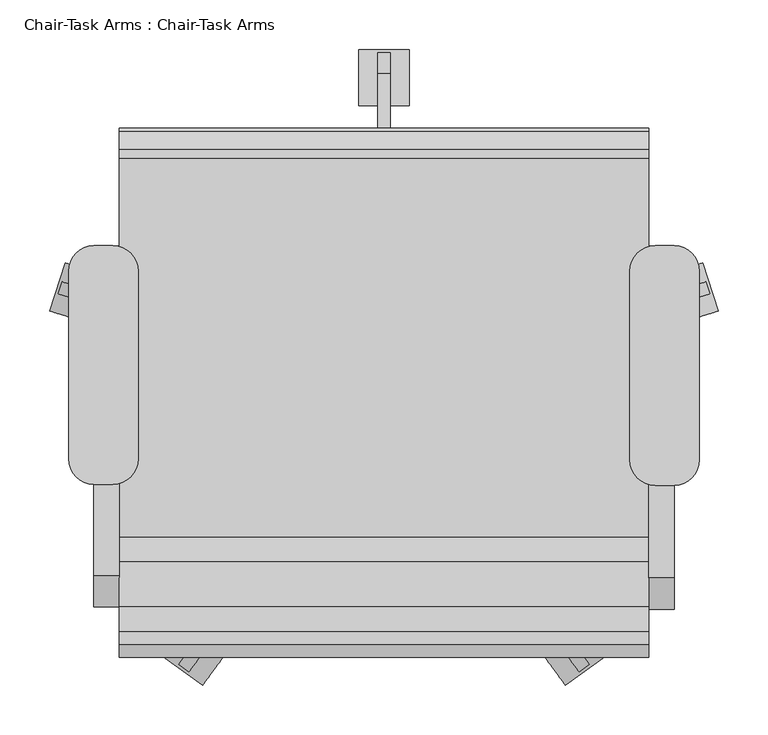
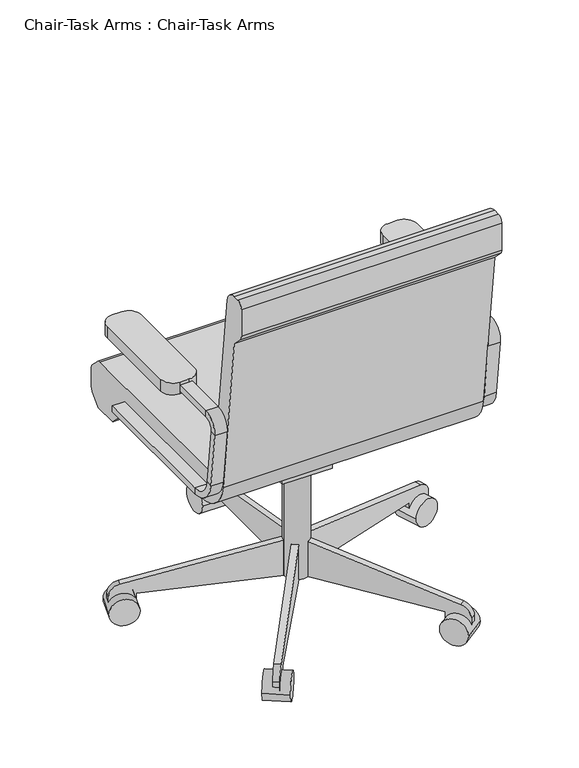
"""IFC4 building model written with IfcOpenShell, lengths in millimetres: furniture geometry, Chair-Task Arms : Chair-Task Arms."""

from ifc_helpers import new_model, si_unit, point, frame, frame_2d, origin, place, context, project, spatial, polyline, circle_curve, trimmed, segment, composite_curve, outline, extrude, source, transform, mapped, element, save
from ifc_brep_helpers import plane_surface, cylinder_surface, revolved_surface, advanced_brep


def chair_task_arms_chair_task_arms_fa5a08ef(model_context):
    return source(origin(), model_context, "Body", "SolidModel", [
        extrude(outline(composite_curve([segment(polyline([(433.0908197, -74.2028048), (414.0408197, -74.2028048)]), True, "CONTINUOUS"), segment(trimmed(circle_curve(frame_2d((414.0408197, -48.8028048)), 25.4), [point((414.0408197, -74.2028048))], [point((388.6408197, -48.8028048))], False, "CARTESIAN"), True, "CONTINUOUS"), segment(polyline([(388.6408197, -48.8028048), (388.6408197, 141.6319091)]), True, "CONTINUOUS"), segment(trimmed(circle_curve(frame_2d((414.0408197, 141.6319091)), 25.4), [point((388.6408197, 141.6319091))], [point((414.0408197, 167.0319091))], False, "CARTESIAN"), True, "CONTINUOUS"), segment(polyline([(414.0408197, 167.0319091), (433.0908197, 167.0319091)]), True, "CONTINUOUS"), segment(trimmed(circle_curve(frame_2d((433.0908197, 141.6319091)), 25.4), [point((433.0908197, 167.0319091))], [point((458.4908197, 141.6319091))], False, "CARTESIAN"), True, "CONTINUOUS"), segment(polyline([(458.4908197, 141.6319091), (458.4908197, -48.8028048)]), True, "CONTINUOUS"), segment(trimmed(circle_curve(frame_2d((433.0908197, -48.8028048)), 25.4), [point((458.4908197, -48.8028048))], [point((433.0908197, -74.2028048))], False, "CARTESIAN"), True, "CONTINUOUS")], self_intersect=False)), frame((0.0, 0.0, 596.9), z_axis=(0.0, 0.0, 1.0), x_axis=(1.0, 0.0, 0.0)), (0.0, 0.0, 1.0), 25.4),
        extrude(outline(composite_curve([segment(polyline([(-132.0591803, -73.1575984), (-151.1091803, -73.1575984)]), True, "CONTINUOUS"), segment(trimmed(circle_curve(frame_2d((-151.1091803, -47.7575984)), 25.4), [point((-151.1091803, -73.1575984))], [point((-176.5091803, -47.7575984))], False, "CARTESIAN"), True, "CONTINUOUS"), segment(polyline([(-176.5091803, -47.7575984), (-176.5091803, 141.6319091)]), True, "CONTINUOUS"), segment(trimmed(circle_curve(frame_2d((-151.1091803, 141.6319091)), 25.4), [point((-176.5091803, 141.6319091))], [point((-151.1091803, 167.0319091))], False, "CARTESIAN"), True, "CONTINUOUS"), segment(polyline([(-151.1091803, 167.0319091), (-132.0591803, 167.0319091)]), True, "CONTINUOUS"), segment(trimmed(circle_curve(frame_2d((-132.0591803, 141.6319091)), 25.4), [point((-132.0591803, 167.0319091))], [point((-106.6591803, 141.6319091))], False, "CARTESIAN"), True, "CONTINUOUS"), segment(polyline([(-106.6591803, 141.6319091), (-106.6591803, -47.7575984)]), True, "CONTINUOUS"), segment(trimmed(circle_curve(frame_2d((-132.0591803, -47.7575984)), 25.4), [point((-106.6591803, -47.7575984))], [point((-132.0591803, -73.1575984))], False, "CARTESIAN"), True, "CONTINUOUS")], self_intersect=False)), frame((0.0, 0.0, 596.9), z_axis=(0.0, 0.0, 1.0), x_axis=(1.0, 0.0, 0.0)), (0.0, 0.0, 1.0), 25.4),
        advanced_brep(
        [(-151.1091803, 167.0319091, 412.75), (-151.1091803, 167.0319091, 425.45), (-125.7091803, 167.0319091, 425.45), (-125.7091803, 167.0319091, 412.75), (-151.1091803, -126.2388651, 412.75), (-151.1091803, -126.2388651, 425.45), (-125.7091803, -126.2388651, 425.45), (-125.7091803, -126.2388651, 412.75), (-151.1091803, -170.3844094, 464.7064065), (-151.1091803, -182.9974221, 463.2225227), (-125.7091803, -170.3844094, 464.7064065), (-125.7091803, -182.9974221, 463.2225227), (-151.1091803, -196.7936301, 580.4902904), (-151.1091803, -184.1806174, 581.9741742), (-125.7091803, -184.1806174, 581.9741742), (-125.7091803, -196.7936301, 580.4902904), (-151.1091803, -165.2610984, 603.25), (-151.1091803, -165.2610984, 615.95), (-125.7091803, -165.2610984, 603.25), (-125.7091803, -165.2610984, 615.95), (-151.1091803, 18.9459016, 615.95), (-125.7091803, 18.9459016, 615.95), (-125.7091803, 18.9459016, 603.25), (-151.1091803, 18.9459016, 603.25)],
        [
            (0, 1),
            (1, 2),
            (2, 3),
            (3, 0),
            (0, 4),
            (4, 5),
            (5, 1),
            (5, 6),
            (6, 2),
            (6, 7),
            (7, 3),
            (7, 4),
            (8, 5, circle_curve(frame((-151.1091803, -126.2388651, 469.9), z_axis=(1.0, 0.0, 0.0), x_axis=(0.0, 0.0, -1.0)), 44.45)),
            (4, 9, circle_curve(frame((-151.1091803, -126.2388651, 469.9), z_axis=(-1.0, 0.0, 0.0), x_axis=(0.0, 0.0, -1.0)), 57.15)),
            (9, 8),
            (10, 6, circle_curve(frame((-125.7091803, -126.2388651, 469.9), z_axis=(1.0, 0.0, 0.0), x_axis=(0.0, 0.0, -1.0)), 44.45)),
            (8, 10),
            (11, 7, circle_curve(frame((-125.7091803, -126.2388651, 469.9), z_axis=(1.0, 0.0, 0.0), x_axis=(0.0, 0.0, -1.0)), 57.15)),
            (10, 11),
            (11, 9),
            (9, 12),
            (12, 13),
            (13, 8),
            (13, 14),
            (14, 10),
            (14, 15),
            (15, 11),
            (15, 12),
            (16, 13, circle_curve(frame((-151.1091803, -165.2610984, 584.2), z_axis=(1.0, 0.0, 0.0), x_axis=(0.0, -0.9931506043228768, -0.11684124756739202)), 19.05)),
            (12, 17, circle_curve(frame((-151.1091803, -165.2610984, 584.2), z_axis=(-1.0, 0.0, 0.0), x_axis=(0.0, -0.9931506043228768, -0.11684124756739202)), 31.75)),
            (17, 16),
            (18, 14, circle_curve(frame((-125.7091803, -165.2610984, 584.2), z_axis=(1.0, 0.0, 0.0), x_axis=(0.0, -0.9931506043228768, -0.11684124756739202)), 19.05)),
            (16, 18),
            (19, 15, circle_curve(frame((-125.7091803, -165.2610984, 584.2), z_axis=(1.0, 0.0, 0.0), x_axis=(0.0, -0.9931506043228768, -0.11684124756739202)), 31.75)),
            (18, 19),
            (19, 17),
            (20, 21),
            (21, 22),
            (22, 23),
            (23, 20),
            (17, 20),
            (23, 16),
            (22, 18),
            (21, 19),
        ],
        [
            plane_surface(frame((-152.608212, 167.0319091, 419.1), z_axis=(0.0, 1.0, 0.0), x_axis=(0.0, 0.0, -1.0))),
            plane_surface(frame((-151.1091803, 167.0319091, 412.75), z_axis=(-1.0, 0.0, 0.0), x_axis=(0.0, -1.0, 0.0))),
            plane_surface(frame((-151.1091803, 167.0319091, 425.45), z_axis=(0.0, 0.0, 1.0), x_axis=(0.0, -1.0, 0.0))),
            plane_surface(frame((-125.7091803, 167.0319091, 425.45), z_axis=(1.0, 0.0, 0.0), x_axis=(0.0, -1.0, 0.0))),
            plane_surface(frame((-125.7091803, 167.0319091, 412.75), z_axis=(0.0, 0.0, -1.0), x_axis=(0.0, -1.0, 0.0))),
            plane_surface(frame((-151.1091803, -126.2388651, 469.9), z_axis=(-1.0, 0.0, 0.0), x_axis=(0.0, 0.0, -1.0))),
            revolved_surface(polyline([(-151.1091803, -126.2388651, 425.45), (-125.7091803, -126.2388651, 425.45)]), (-138.4091803, -126.2388651, 469.9), (-1.0, 0.0, 0.0)),
            plane_surface(frame((-125.7091803, -126.2388651, 469.9), z_axis=(1.0, 0.0, 0.0), x_axis=(0.0, 0.0, -1.0))),
            cylinder_surface(frame((-138.4091803, -126.2388651, 469.9), z_axis=(-1.0, 0.0, 0.0), x_axis=(0.0, 0.0, -1.0)), 57.15),
            plane_surface(frame((-151.1091803, -182.9974221, 463.2225227), z_axis=(-1.0, 0.0, 0.0), x_axis=(0.0, -0.1168412475673856, 0.9931506043228776))),
            plane_surface(frame((-151.1091803, -170.3844094, 464.7064065), z_axis=(0.0, 0.9931506043228776, 0.1168412475673856), x_axis=(0.0, -0.1168412475673856, 0.9931506043228776))),
            plane_surface(frame((-125.7091803, -170.3844094, 464.7064065), z_axis=(1.0, 0.0, 0.0), x_axis=(0.0, -0.1168412475673856, 0.9931506043228776))),
            plane_surface(frame((-125.7091803, -182.9974221, 463.2225227), z_axis=(0.0, -0.9931506043228776, -0.1168412475673856), x_axis=(0.0, -0.1168412475673856, 0.9931506043228776))),
            plane_surface(frame((-151.1091803, -165.2610984, 584.2), z_axis=(-1.0, 0.0, 0.0), x_axis=(0.0, -0.9931506043228768, -0.11684124756739202))),
            revolved_surface(polyline([(-151.1091803, -184.1806174123508, 581.9741742338413), (-125.7091803, -184.1806174123508, 581.9741742338413)]), (-138.4091803, -165.2610984, 584.2), (-1.0, 0.0, 0.0)),
            plane_surface(frame((-125.7091803, -165.2610984, 584.2), z_axis=(1.0, 0.0, 0.0), x_axis=(0.0, -0.9931506043228768, -0.11684124756739202))),
            cylinder_surface(frame((-138.4091803, -165.2610984, 584.2), z_axis=(-1.0, 0.0, 0.0), x_axis=(0.0, -0.9931506043228768, -0.11684124756739202)), 31.75),
            plane_surface(frame((-152.608212, 18.9459016, 609.6), z_axis=(0.0, 1.0, 0.0), x_axis=(0.0, 0.0, 1.0))),
            plane_surface(frame((-151.1091803, -165.2610984, 615.95), z_axis=(-1.0, 0.0, 0.0), x_axis=(0.0, 1.0, 0.0))),
            plane_surface(frame((-151.1091803, -165.2610984, 603.25), z_axis=(0.0, 0.0, -1.0), x_axis=(0.0, 1.0, 0.0))),
            plane_surface(frame((-125.7091803, -165.2610984, 603.25), z_axis=(1.0, 0.0, 0.0), x_axis=(0.0, 1.0, 0.0))),
            plane_surface(frame((-125.7091803, -165.2610984, 615.95), z_axis=(0.0, 0.0, 1.0), x_axis=(0.0, 1.0, 0.0))),
        ],
        [
            (0, [[1, 2, 3, 4]]),
            (1, [[-1, 5, 6, 7]]),
            (2, [[-2, -7, 8, 9]]),
            (3, [[-3, -9, 10, 11]]),
            (4, [[-4, -11, 12, -5]]),
            (5, [[13, -6, 14, 15]]),
            (6, [[16, -8, -13, 17]]),
            (7, [[18, -10, -16, 19]]),
            (8, [[-14, -12, -18, 20]]),
            (9, [[-15, 21, 22, 23]]),
            (10, [[-17, -23, 24, 25]]),
            (11, [[-19, -25, 26, 27]]),
            (12, [[-20, -27, 28, -21]]),
            (13, [[29, -22, 30, 31]]),
            (14, [[32, -24, -29, 33]]),
            (15, [[34, -26, -32, 35]]),
            (16, [[-30, -28, -34, 36]]),
            (17, [[37, 38, 39, 40]]),
            (18, [[-31, 41, -40, 42]]),
            (19, [[-33, -42, -39, 43]]),
            (20, [[-35, -43, -38, 44]]),
            (21, [[-36, -44, -37, -41]]),
        ],
    ),
        advanced_brep(
        [(433.0908197, 167.0319091, 425.45), (433.0908197, 167.0319091, 412.75), (407.6908197, 167.0319091, 412.75), (407.6908197, 167.0319091, 425.45), (433.0908197, -128.329278, 425.45), (433.0908197, -128.329278, 412.75), (407.6908197, -128.329278, 412.75), (407.6908197, -128.329278, 425.45), (433.0908197, -185.0878351, 463.2225227), (433.0908197, -172.4748224, 464.7064065), (407.6908197, -185.0878351, 463.2225227), (407.6908197, -172.4748224, 464.7064065), (433.0908197, -186.2710303, 581.9741742), (433.0908197, -198.884043, 580.4902904), (407.6908197, -198.884043, 580.4902904), (407.6908197, -186.2710303, 581.9741742), (433.0908197, -167.3515113, 615.95), (433.0908197, -167.3515113, 603.25), (407.6908197, -167.3515113, 615.95), (407.6908197, -167.3515113, 603.25), (433.0908197, 18.9459016, 603.25), (407.6908197, 18.9459016, 603.25), (407.6908197, 18.9459016, 615.95), (433.0908197, 18.9459016, 615.95)],
        [
            (0, 1),
            (1, 2),
            (2, 3),
            (3, 0),
            (0, 4),
            (4, 5),
            (5, 1),
            (5, 6),
            (6, 2),
            (6, 7),
            (7, 3),
            (7, 4),
            (8, 5, circle_curve(frame((433.0908197, -128.329278, 469.9), z_axis=(1.0, 0.0, 0.0), x_axis=(0.0, 0.0, -1.0)), 57.15)),
            (4, 9, circle_curve(frame((433.0908197, -128.329278, 469.9), z_axis=(-1.0, 0.0, 0.0), x_axis=(0.0, 0.0, -1.0)), 44.45)),
            (9, 8),
            (10, 6, circle_curve(frame((407.6908197, -128.329278, 469.9), z_axis=(1.0, 0.0, 0.0), x_axis=(0.0, 0.0, -1.0)), 57.15)),
            (8, 10),
            (11, 7, circle_curve(frame((407.6908197, -128.329278, 469.9), z_axis=(1.0, 0.0, 0.0), x_axis=(0.0, 0.0, -1.0)), 44.45)),
            (10, 11),
            (11, 9),
            (9, 12),
            (12, 13),
            (13, 8),
            (13, 14),
            (14, 10),
            (14, 15),
            (15, 11),
            (15, 12),
            (16, 13, circle_curve(frame((433.0908197, -167.3515113, 584.2), z_axis=(1.0, 0.0, 0.0), x_axis=(0.0, -0.9931506043228767, -0.1168412475673929)), 31.75)),
            (12, 17, circle_curve(frame((433.0908197, -167.3515113, 584.2), z_axis=(-1.0, 0.0, 0.0), x_axis=(0.0, -0.9931506043228767, -0.1168412475673929)), 19.05)),
            (17, 16),
            (18, 14, circle_curve(frame((407.6908197, -167.3515113, 584.2), z_axis=(1.0, 0.0, 0.0), x_axis=(0.0, -0.9931506043228767, -0.1168412475673929)), 31.75)),
            (16, 18),
            (19, 15, circle_curve(frame((407.6908197, -167.3515113, 584.2), z_axis=(1.0, 0.0, 0.0), x_axis=(0.0, -0.9931506043228767, -0.1168412475673929)), 19.05)),
            (18, 19),
            (19, 17),
            (20, 21),
            (21, 22),
            (22, 23),
            (23, 20),
            (17, 20),
            (23, 16),
            (22, 18),
            (21, 19),
        ],
        [
            plane_surface(frame((406.191788, 167.0319091, 419.1), z_axis=(0.0, 1.0, 0.0), x_axis=(0.0, 0.0, -1.0))),
            plane_surface(frame((433.0908197, 167.0319091, 425.45), z_axis=(1.0, 0.0, 0.0), x_axis=(0.0, -1.0, 0.0))),
            plane_surface(frame((433.0908197, 167.0319091, 412.75), z_axis=(0.0, 0.0, -1.0), x_axis=(0.0, -1.0, 0.0))),
            plane_surface(frame((407.6908197, 167.0319091, 412.75), z_axis=(-1.0, 0.0, 0.0), x_axis=(0.0, -1.0, 0.0))),
            plane_surface(frame((407.6908197, 167.0319091, 425.45), z_axis=(0.0, 0.0, 1.0), x_axis=(0.0, -1.0, 0.0))),
            plane_surface(frame((433.0908197, -128.329278, 469.9), z_axis=(1.0, 0.0, 0.0), x_axis=(0.0, 0.0, -1.0))),
            cylinder_surface(frame((420.3908197, -128.329278, 469.9), z_axis=(-1.0, 0.0, 0.0), x_axis=(0.0, 0.0, -1.0)), 57.15),
            plane_surface(frame((407.6908197, -128.329278, 469.9), z_axis=(-1.0, 0.0, 0.0), x_axis=(0.0, 0.0, -1.0))),
            revolved_surface(polyline([(407.6908197, -128.329278, 425.45), (433.0908197, -128.329278, 425.45)]), (420.3908197, -128.329278, 469.9), (-1.0, 0.0, 0.0)),
            plane_surface(frame((433.0908197, -172.4748224, 464.7064065), z_axis=(1.0, 0.0, 0.0), x_axis=(0.0, -0.11684124756738626, 0.9931506043228775))),
            plane_surface(frame((433.0908197, -185.0878351, 463.2225227), z_axis=(0.0, -0.9931506043228775, -0.11684124756738655), x_axis=(0.0, -0.11684124756738655, 0.9931506043228775))),
            plane_surface(frame((407.6908197, -185.0878351, 463.2225227), z_axis=(-1.0, 0.0, 0.0), x_axis=(0.0, -0.11684124756738626, 0.9931506043228775))),
            plane_surface(frame((407.6908197, -172.4748224, 464.7064065), z_axis=(0.0, 0.9931506043228775, 0.11684124756738626), x_axis=(0.0, -0.11684124756738626, 0.9931506043228775))),
            plane_surface(frame((433.0908197, -167.3515113, 584.2), z_axis=(1.0, 0.0, 0.0), x_axis=(0.0, -0.9931506043228767, -0.1168412475673929))),
            cylinder_surface(frame((420.3908197, -167.3515113, 584.2), z_axis=(-1.0, 0.0, 0.0), x_axis=(0.0, -0.9931506043228767, -0.1168412475673929)), 31.75),
            plane_surface(frame((407.6908197, -167.3515113, 584.2), z_axis=(-1.0, 0.0, 0.0), x_axis=(0.0, -0.9931506043228767, -0.1168412475673929))),
            revolved_surface(polyline([(407.6908197, -186.2710303123508, 581.9741742338412), (433.0908197, -186.2710303123508, 581.9741742338412)]), (420.3908197, -167.3515113, 584.2), (-1.0, 0.0, 0.0)),
            plane_surface(frame((406.191788, 18.9459016, 609.6), z_axis=(0.0, 1.0, 0.0), x_axis=(0.0, 0.0, 1.0))),
            plane_surface(frame((433.0908197, -167.3515113, 603.25), z_axis=(1.0, 0.0, 0.0), x_axis=(0.0, 1.0, 0.0))),
            plane_surface(frame((433.0908197, -167.3515113, 615.95), z_axis=(0.0, 0.0, 1.0), x_axis=(0.0, 1.0, 0.0))),
            plane_surface(frame((407.6908197, -167.3515113, 615.95), z_axis=(-1.0, 0.0, 0.0), x_axis=(0.0, 1.0, 0.0))),
            plane_surface(frame((407.6908197, -167.3515113, 603.25), z_axis=(0.0, 0.0, -1.0), x_axis=(0.0, 1.0, 0.0))),
        ],
        [
            (0, [[1, 2, 3, 4]]),
            (1, [[-1, 5, 6, 7]]),
            (2, [[-2, -7, 8, 9]]),
            (3, [[-3, -9, 10, 11]]),
            (4, [[-4, -11, 12, -5]]),
            (5, [[13, -6, 14, 15]]),
            (6, [[16, -8, -13, 17]]),
            (7, [[18, -10, -16, 19]]),
            (8, [[-14, -12, -18, 20]]),
            (9, [[-15, 21, 22, 23]]),
            (10, [[-17, -23, 24, 25]]),
            (11, [[-19, -25, 26, 27]]),
            (12, [[-20, -27, 28, -21]]),
            (13, [[29, -22, 30, 31]]),
            (14, [[32, -24, -29, 33]]),
            (15, [[34, -26, -32, 35]]),
            (16, [[-30, -28, -34, 36]]),
            (17, [[37, 38, 39, 40]]),
            (18, [[-31, 41, -40, 42]]),
            (19, [[-33, -42, -39, 43]]),
            (20, [[-35, -43, -38, 44]]),
            (21, [[-36, -44, -37, -41]]),
        ],
    ),
        extrude(outline(composite_curve([segment(trimmed(circle_curve(frame_2d((140.9908197, 18.9459016)), 25.4), [point((115.5908197, 18.9459016))], [point((166.3908197, 18.9459016))], False, "CARTESIAN"), True, "CONTINUOUS"), segment(trimmed(circle_curve(frame_2d((140.9908197, 18.9459016)), 25.4), [point((166.3908197, 18.9459016))], [point((115.5908197, 18.9459016))], False, "CARTESIAN"), True, "CONTINUOUS")], self_intersect=False)), frame((0.0, 0.0, 53.5835944), z_axis=(0.0, 0.0, 1.0), x_axis=(1.0, 0.0, 0.0)), (0.0, 0.0, 1.0), 330.5914056),
        extrude(outline(composite_curve([segment(trimmed(circle_curve(frame_2d((0.0, -28.2002727)), 28.2002727), [point((0.0, -56.4005455))], [point((0.0, 0.0))], False, "CARTESIAN"), True, "CONTINUOUS"), segment(trimmed(circle_curve(frame_2d((0.0, -28.2002727)), 28.2002727), [point((0.0, 0.0))], [point((0.0, -56.4005455))], False, "CARTESIAN"), True, "CONTINUOUS")], self_intersect=False)), frame((477.6203484, 101.6163254, 28.1835944), z_axis=(-0.3090169943749423, 0.9510565162951553, 0.0), x_axis=(0.0, 0.0, 1.0)), (0.0, 0.0, 1.0), 50.8),
        extrude(outline(composite_curve([segment(polyline([(-25.4, 0.0), (0.0, 0.0), (0.0, -50.8), (-24.303053, -50.8)]), True, "CONTINUOUS"), segment(trimmed(circle_curve(frame_2d((-24.303053, -25.4)), 25.4), [point((-24.303053, -50.8))], [point((-49.3171699, -29.8106637))], False, "CARTESIAN"), True, "CONTINUOUS"), segment(polyline([(-49.3171699, -29.8106637), (-101.6, 266.7), (-101.6, 292.1), (-25.4, 292.1), (-25.4, 0.0)]), True, "CONTINUOUS")], self_intersect=False)), frame((420.756686, 103.1705568, 28.1835944), z_axis=(-0.3090169943749423, 0.9510565162951553, 0.0), x_axis=(0.0, 0.0, -1.0)), (0.0, 0.0, 1.0), 12.7),
        extrude(outline(composite_curve([segment(trimmed(circle_curve(frame_2d((0.0, -28.2002727)), 28.2002727), [point((0.0, -56.4005455))], [point((0.0, 0.0))], False, "CARTESIAN"), True, "CONTINUOUS"), segment(trimmed(circle_curve(frame_2d((0.0, -28.2002727)), 28.2002727), [point((0.0, 0.0))], [point((0.0, -56.4005455))], False, "CARTESIAN"), True, "CONTINUOUS")], self_intersect=False)), frame((323.63931, -275.6612394, 28.1835944), z_axis=(0.8090169943749499, 0.5877852522924699, 0.0), x_axis=(0.0, 0.0, 1.0)), (0.0, 0.0, 1.0), 50.8),
        extrude(outline(composite_curve([segment(polyline([(-25.4, 0.0), (0.0, 0.0), (0.0, -50.8), (-24.303053, -50.8)]), True, "CONTINUOUS"), segment(trimmed(circle_curve(frame_2d((-24.303053, -25.3999999)), 25.4), [point((-24.303053, -50.8))], [point((-49.3171699, -29.8106636))], False, "CARTESIAN"), True, "CONTINUOUS"), segment(polyline([(-49.3171699, -29.8106636), (-101.6, 266.7), (-101.6, 292.1), (-25.4, 292.1), (-25.4, 0.0)]), True, "CONTINUOUS")], self_intersect=False)), frame((307.545634, -221.1003988, 28.1835944), z_axis=(0.8090169943749499, 0.5877852522924699, 0.0), x_axis=(0.0, 0.0, -1.0)), (0.0, 0.0, 1.0), 12.7),
        extrude(outline(composite_curve([segment(trimmed(circle_curve(frame_2d((0.0, -28.2002727)), 28.2002727), [point((0.0, -56.4005455))], [point((0.0, 0.0))], False, "CARTESIAN"), True, "CONTINUOUS"), segment(trimmed(circle_curve(frame_2d((0.0, -28.2002727)), 28.2002727), [point((0.0, 0.0))], [point((0.0, -56.4005455))], False, "CARTESIAN"), True, "CONTINUOUS")], self_intersect=False)), frame((-41.6576707, -275.6612394, 28.1835944), z_axis=(-0.8090169943749458, 0.5877852522924754, 0.0), x_axis=(0.0, 0.0, -1.0)), (0.0, 0.0, 1.0), 50.8),
        extrude(outline(composite_curve([segment(polyline([(25.4, 0.0), (25.4, 292.1), (101.6, 292.1), (101.6, 266.7), (49.3171699, -29.8106637)]), True, "CONTINUOUS"), segment(trimmed(circle_curve(frame_2d((24.303053, -25.3999999)), 25.4), [point((49.3171699, -29.8106637))], [point((24.303053, -50.8))], False, "CARTESIAN"), True, "CONTINUOUS"), segment(polyline([(24.303053, -50.8), (0.0, -50.8), (0.0, 0.0), (25.4, 0.0)]), True, "CONTINUOUS")], self_intersect=False)), frame((-25.5639946, -221.1003988, 28.1835944), z_axis=(-0.8090169943749459, 0.5877852522924754, 0.0), x_axis=(0.0, 0.0, 1.0)), (0.0, 0.0, 1.0), 12.7),
        extrude(outline(composite_curve([segment(trimmed(circle_curve(frame_2d((0.0, -28.2002727)), 28.2002727), [point((0.0, -56.4005454))], [point((0.0, 0.0))], False, "CARTESIAN"), True, "CONTINUOUS"), segment(trimmed(circle_curve(frame_2d((0.0, -28.2002727)), 28.2002727), [point((0.0, 0.0))], [point((0.0, -56.4005454))], False, "CARTESIAN"), True, "CONTINUOUS")], self_intersect=False)), frame((-195.638709, 101.6163254, 28.1835944), z_axis=(0.3090169943749487, 0.9510565162951532, 0.0), x_axis=(0.0, 0.0, -1.0)), (0.0, 0.0, 1.0), 50.8),
        extrude(outline(composite_curve([segment(polyline([(25.4, 0.0), (25.4, 292.1000001), (101.6, 292.1000001), (101.6, 266.7), (49.3171699, -29.8106636)]), True, "CONTINUOUS"), segment(trimmed(circle_curve(frame_2d((24.303053, -25.4)), 25.4), [point((49.3171699, -29.8106636))], [point((24.303053, -50.8))], False, "CARTESIAN"), True, "CONTINUOUS"), segment(polyline([(24.303053, -50.8), (0.0, -50.8), (0.0, 0.0), (25.4, 0.0)]), True, "CONTINUOUS")], self_intersect=False)), frame((-138.7750467, 103.1705568, 28.1835944), z_axis=(0.3090169943749487, 0.9510565162951532, 0.0), x_axis=(0.0, 0.0, 1.0)), (0.0, 0.0, 1.0), 12.7),
        extrude(outline(composite_curve([segment(trimmed(circle_curve(frame_2d((336.4459016, 28.1835944)), 28.2002727), [point((308.2456289, 28.1835944))], [point((364.6461744, 28.1835944))], False, "CARTESIAN"), True, "CONTINUOUS"), segment(trimmed(circle_curve(frame_2d((336.4459016, 28.1835944)), 28.2002727), [point((364.6461744, 28.1835944))], [point((308.2456289, 28.1835944))], False, "CARTESIAN"), True, "CONTINUOUS")], self_intersect=False)), frame((115.5908197, 0.0, 0.0), z_axis=(1.0, 0.0, 0.0), x_axis=(0.0, 1.0, 0.0)), (0.0, 0.0, 1.0), 50.8),
        extrude(outline(composite_curve([segment(polyline([(311.0459016, 53.5835944), (18.9459016, 53.5835944), (18.9459016, 129.7835944), (44.3459016, 129.7835944), (340.8565654, 77.5007643)]), True, "CONTINUOUS"), segment(trimmed(circle_curve(frame_2d((336.4459016, 52.4866474)), 25.4), [point((340.8565654, 77.5007643))], [point((361.8459016, 52.4866474))], False, "CARTESIAN"), True, "CONTINUOUS"), segment(polyline([(361.8459016, 52.4866474), (361.8459016, 28.1835944), (311.0459016, 28.1835944), (311.0459016, 53.5835944)]), True, "CONTINUOUS")], self_intersect=False)), frame((134.6408197, 0.0, 0.0), z_axis=(1.0, 0.0, 0.0), x_axis=(0.0, 1.0, 0.0)), (0.0, 0.0, 1.0), 12.7),
        extrude(outline(polyline([(69.7459016, 383.7835944), (69.7459016, 371.0835944), (18.9459016, 283.0954134), (-19.1540984, 283.0954134), (-19.1540984, 383.7835944), (69.7459016, 383.7835944)])), frame((90.1908197, 0.0, 0.0), z_axis=(1.0, 0.0, 0.0), x_axis=(0.0, 1.0, 0.0)), (0.0, 0.0, 1.0), 101.6),
        extrude(outline(composite_curve([segment(polyline([(-126.2050455, 457.2), (255.0102301, 457.2)]), True, "CONTINUOUS"), segment(trimmed(circle_curve(frame_2d((255.0102301, 444.5)), 12.7), [point((255.0102301, 457.2))], [point((263.9604301, 453.510212))], False, "CARTESIAN"), True, "CONTINUOUS"), segment(polyline([(263.9604301, 453.510212), (281.8961016, 435.6939999)]), True, "CONTINUOUS"), segment(trimmed(circle_curve(frame_2d((272.9459016, 426.6837879)), 12.7), [point((281.8961016, 435.6939999))], [point((285.6459016, 426.6837879))], False, "CARTESIAN"), True, "CONTINUOUS"), segment(polyline([(285.6459016, 426.6837879), (285.6459016, 391.6405184)]), True, "CONTINUOUS"), segment(trimmed(circle_curve(frame_2d((260.2459016, 391.6405184)), 25.4), [point((285.6459016, 391.6405184))], [point((278.2663256, 373.7401184))], False, "CARTESIAN"), True, "CONTINUOUS"), segment(polyline([(278.2663256, 373.7401184), (260.2470284, 355.6), (209.4470284, 355.6), (181.0744602, 383.7835944), (-107.1089978, 383.7835944)]), True, "CONTINUOUS"), segment(trimmed(circle_curve(frame_2d((-107.1089978, 459.9835944)), 76.2), [point((-107.1089978, 383.7835944))], [point((-182.7870738, 451.0802913))], False, "CARTESIAN"), True, "CONTINUOUS"), segment(polyline([(-182.7870738, 451.0802913), (-222.3540984, 787.4), (-244.0343545, 809.0802561)]), True, "CONTINUOUS"), segment(trimmed(circle_curve(frame_2d((-235.0540984, 818.0605122)), 12.7), [point((-244.0343545, 809.0802561))], [point((-247.7540984, 818.0605122))], False, "CARTESIAN"), True, "CONTINUOUS"), segment(polyline([(-247.7540984, 818.0605122), (-247.7540984, 876.3)]), True, "CONTINUOUS"), segment(trimmed(circle_curve(frame_2d((-235.0540984, 876.3)), 12.7), [point((-247.7540984, 876.3))], [point((-235.0540984, 889.0))], False, "CARTESIAN"), True, "CONTINUOUS"), segment(polyline([(-235.0540984, 889.0), (-222.1789239, 889.0)]), True, "CONTINUOUS"), segment(trimmed(circle_curve(frame_2d((-222.1789239, 863.6)), 25.4), [point((-222.1789239, 889.0))], [point((-196.9528985, 866.5677677))], False, "CARTESIAN"), True, "CONTINUOUS"), segment(polyline([(-196.9528985, 866.5677677), (-151.4310708, 479.6322323)]), True, "CONTINUOUS"), segment(trimmed(circle_curve(frame_2d((-126.2050455, 482.6)), 25.4), [point((-151.4310708, 479.6322323))], [point((-126.2050455, 457.2))], True, "CARTESIAN"), True, "CONTINUOUS")], self_intersect=False)), frame((-125.7091803, 0.0, 0.0), z_axis=(1.0, 0.0, 0.0), x_axis=(0.0, 1.0, 0.0)), (0.0, 0.0, 1.0), 533.4),
    ])


if __name__ == "__main__":
    model = new_model("IFC4")
    model_context = context("Model", 3, world=origin())
    ifc_project = project(units=[si_unit("LENGTHUNIT", "METRE", prefix="MILLI")], contexts=[model_context])
    site = spatial("IfcSite", under=ifc_project)
    building = spatial("IfcBuilding", under=site)
    placement = place(None, origin())
    chair_task_arms_chair_task_arms_shape = chair_task_arms_chair_task_arms_fa5a08ef(model_context)
    element("IfcFurniture", 1, ObjectType="Chair-Task Arms : Chair-Task Arms", at=placement, inside=building, context=model_context, shape_type="MappedRepresentation", body=[
        mapped(chair_task_arms_chair_task_arms_shape, transform((0.0, 0.0, 0.0), x_axis=(1.0, 0.0, 0.0), y_axis=(0.0, 1.0, 0.0), z_axis=(0.0, 0.0, 1.0))),
    ])
    save(model, "model.ifc")

# Revit data of these elements
# Type "Chair-Task Arms : Chair-Task Arms"
#   Assembly Code = "E2020200"
#   Base Material = Plastic, Opaque Black
#   Caster Material = Plastic, Opaque Black
#   Seat/Back Material = Textile - Slate Blue
#   Default Elevation = 0
# Element 1 (IfcFurniture, "Chair-Task Arms : Chair-Task Arms")
#   Materials on its faces: "Plastic, Opaque Black", "Textile - Slate Blue"
# Materials
#   "Plastic, Opaque Black": class "Plastic", colour RGB 0 0 0, transparency 0.05, Description = "Plastic, generic, opaque black", Cost = 0
#   "Textile - Slate Blue": class "Fabric", colour RGB 98 102 118, transparency 0
